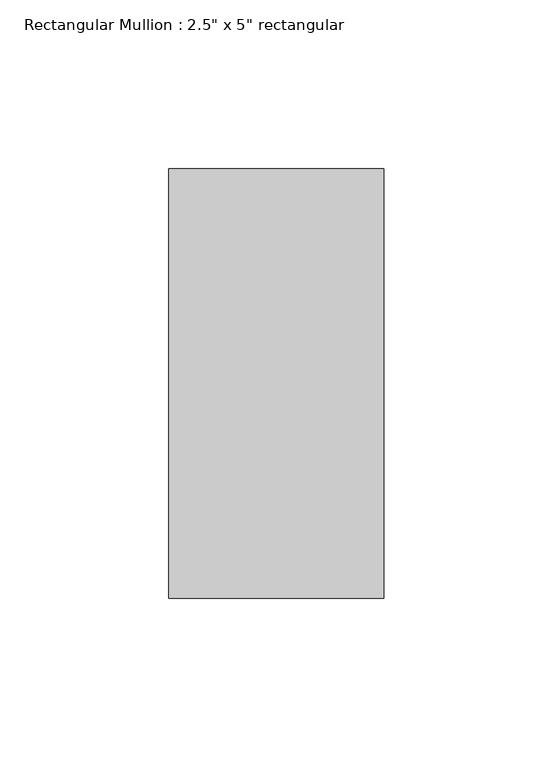
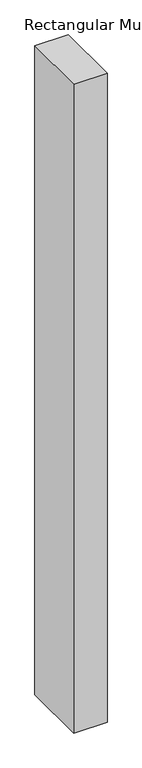
"""IFC4 building model written with IfcOpenShell, lengths in millimetres: member geometry."""

from ifc_helpers import new_model, si_unit, frame, origin, place, context, project, spatial, polyline, outline, extrude, source, transform, mapped, element, save


def member_477baa08(model_context):
    return source(origin(), model_context, "Body", "SweptSolid", [
        extrude(outline(polyline([(0.0, 63.5), (0.0, -63.5), (-63.5, -63.5), (-63.5, 63.5), (0.0, 63.5)])), frame((0.0, 0.0, -1301.645932), z_axis=(0.0, 0.0, 1.0), x_axis=(1.0, 0.0, 0.0)), (0.0, 0.0, 1.0), 1301.645932),
    ])


if __name__ == "__main__":
    model = new_model("IFC4")
    model_context = context("Model", 3, world=origin())
    ifc_project = project(units=[si_unit("LENGTHUNIT", "METRE", prefix="MILLI")], contexts=[model_context])
    site = spatial("IfcSite", under=ifc_project)
    building = spatial("IfcBuilding", under=site)
    placement = place(None, origin())
    member_shape = member_477baa08(model_context)
    element("IfcMember", 1, ObjectType="Rectangular Mullion : 2.5\" x 5\" rectangular", at=placement, inside=building, context=model_context, shape_type="MappedRepresentation", body=[
        mapped(member_shape, transform((0.0, 0.0, 0.0), x_axis=(1.0, 0.0, 0.0), y_axis=(0.0, 1.0, 0.0), z_axis=(0.0, 0.0, 1.0))),
    ])
    save(model, "model.ifc")

# Revit data of these elements
# Type "Rectangular Mullion : 2.5\" x 5\" rectangular"
#   built-in parameter 1007304 = 0.416667 (stored number, unit not read)
#   built-in parameter 1007301 = 0.104167 (stored number, unit not read)
#   built-in parameter 1007300 = 0.104167 (stored number, unit not read)
# Element 1 (IfcMember, "Rectangular Mullion : 2.5\" x 5\" rectangular")
#   Materials on its faces: "Aluminum"
# Materials
#   "Aluminum": class "Metal", colour RGB 247 247 247, transparency 0, Description = "Aluminum 6061", Cost = 0
